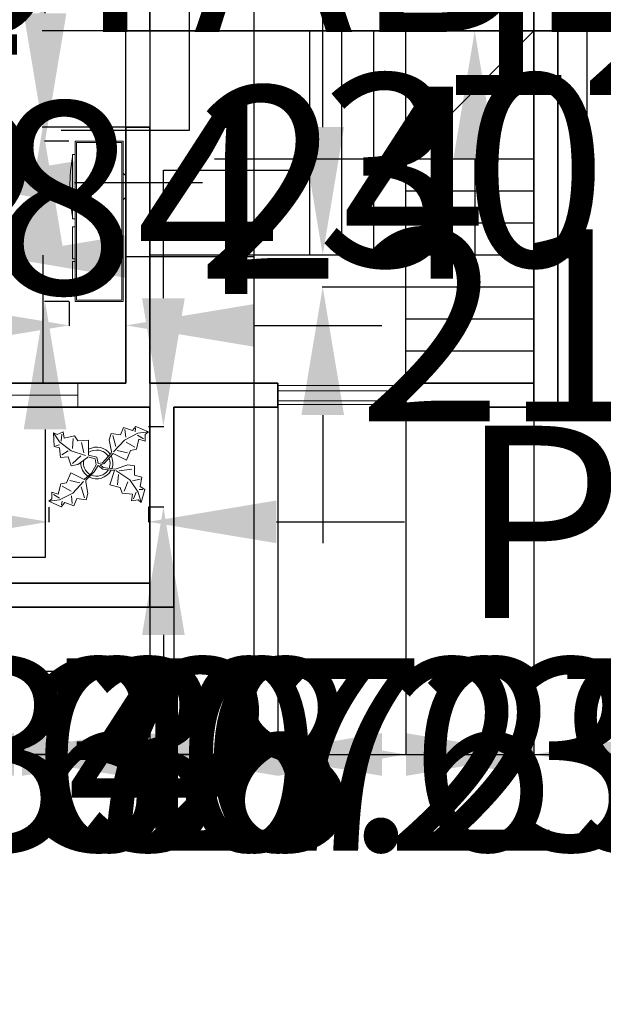
# Model space of a CAD drawing. Units: inches. Extents: x -307 to 2141, y -58 to 895.
# Tile 7 of 28: x 714 to 933, y -58 to 312. Entities that reach past the tile are written whole.
import ezdxf

# ---------------------------------------------------------------- set-up
doc = ezdxf.new("R2010")
doc.units = ezdxf.units.IN
doc.header["$MEASUREMENT"] = 0
for name, color, linetype, lineweight in [('A-ANNO-DIMS', 2, 'Continuous', 18), ('A-FLOR-STRS', 7, 'Continuous', 25), ('A-FURN', 8, 'Continuous', 18), ('A-GLAZ', 4, 'Continuous', 18), ('A-WALL', 7, 'Continuous', 35), ('L-PLNT', 94, 'Continuous', 13)]:
    doc.layers.add(name, color=color, linetype=linetype, lineweight=lineweight)
doc.styles.get("Standard").update_dxf_attribs({"font": 'arial.ttf'})
doc.dimstyles.get("Standard").update_dxf_attribs({"dimtxt": 72, "dimasz": 48, "dimexe": 0.18, "dimexo": 0.0625, "dimgap": 0.09, "dimtad": 0, "dimtih": 1, "dimtoh": 1, "dimdec": 0, "dimrnd": 48, "dimzin": 0, "dimdsep": 46, "dimlunit": 3, "dimtxsty": 'Standard', "dimcen": 0.09, "dimadec": 0, "dimazin": 0, "dimtfac": 1, "dimtdec": 0, "dimtofl": 0, "dimtmove": 0, "dimatfit": 3, "dimfxl": 1, "dimtolj": 1, "dimtzin": 0, "dimarcsym": 0})

# ---------------------------------------------------------------- blocks, each defined once
blk = doc.blocks.new('Entertainment Center')
for p, q in [((-4, 0), (-5, -1)), ((4, 0), (-4, 0)), ((5, -1), (4, 0)), ((-17, -19), (-17, -1)), ((-17, -1), (43, -1)), ((-16.5, -18.5), (-16.5, -1.5)), ((-16.5, -1.5), (42.5, -1.5)), ((42.5, -1.5), (42.5, -18.5)), ((43, -1), (43, -19)), ((43, -19), (-17, -19)), ((42.5, -18.5), (-16.5, -18.5)), ((-12, -20), (-12, -19)), ((12, -20), (-12, -20)), ((12, -19), (12, -20)), ((15, -20), (15, -19)), ((27, -20), (15, -20)), ((27, -19), (27, -20)), ((28, -20), (28, -19)), ((40, -20), (28, -20)), ((40, -19), (40, -20))]:
    blk.add_line(p, q)
blk.add_arc((0, 40), 61, 259.6111, 280.3889)
blk = doc.blocks.new('Plant - Rubber or Philodendron')
for p, q in [((-16.2005, 11.4774), (-13.9899, 8.1064)), ((-16.2005, 11.4774), (-14.8639, 10.7964)), ((-16.0159, 6.3329), (-16.2005, 11.4774)), ((-14.8639, 10.7964), (-12.6195, 11.8975)), ((-12.6195, 11.8975), (-12.1909, 9.4345)), ((4.6914, 8.8812), (5.3859, 11.2828)), ((5.3859, 11.2828), (8.8871, 10.7908)), ((8.8871, 10.7908), (9.9809, 13.4933)), ((9.9809, 13.4933), (13.3837, 12.301)), ((15.3859, 11.3055), (10.3916, 8.7942)), ((10.5828, 12.6946), (10.8893, 9.7953)), ((13.3837, 12.301), (14.68, 13.9039)), ((14.5816, 13.2037), (14.3848, 11.8033)), ((14.68, 13.9039), (19.3848, 11.8146)), ((19.3848, 11.8146), (15.3859, 11.3055)), ((19.3848, 11.8146), (18.1868, 10.9119)), ((-13.9899, 8.1064), (-9.5434, 4.7185)), ((-13.3174, 8.325), (-13.0735, 11.0065)), ((-12.1909, 9.4345), (-8.3829, 10.3)), ((-8.8369, 9.409), (-9.0894, 5.6095)), ((-8.3829, 10.3), (-7.0549, 8.501)), ((-7.0549, 8.501), (-3.0284, 8.6941)), ((-4.8529, 4.012), (-5.7184, 7.82)), ((-3.0284, 8.6941), (-3.0709, 3.1041)), ((4.6914, 8.8812), (5.5014, 4.4831)), ((5.9878, 10.4842), (7.1971, 6.3869)), ((10.3916, 8.7942), (6.2847, 4.4028)), ((14.2977, 6.1031), (10.9934, 7.9956)), ((15.7909, 9.1065), (14.8995, 5.3044)), ((15.2875, 10.6053), (17.5907, 9.2105)), ((18.1925, 8.4119), (15.7909, 9.1065)), ((18.1868, 10.9119), (18.1925, 8.4119)), ((-14.0069, 5.8704), (-16.0159, 6.3329)), ((-15.3434, 6.5514), (-13.9984, 6.9884)), ((-13.5868, 2.2894), (-14.0069, 5.8704)), ((-13.1329, 3.1804), (-10.6614, 4.727)), ((-9.5434, 4.7185), (-4.1917, 2.9888)), ((2.1141, 0.2298), (5.4346, 3.9146)), ((5.4346, 3.9146), (5.5014, 4.4831)), ((7.7005, 4.8881), (11.5025, 3.9967)), ((12.7005, 4.8994), (11.1089, 1.1958)), ((14.8995, 5.3044), (12.7005, 4.8994)), ((-10.6784, 2.491), (-13.5868, 2.2894)), ((-9.5858, -0.8715), (-10.6784, 2.491)), ((-9.1318, 0.0195), (-5.9793, 2.9025)), ((-7.1228, -0.443), (-3.5248, 2.2131)), ((-3.5248, 2.2131), (-3.3011, 2.4355)), ((-3.3011, 2.4355), (-0.5306, 1.7947)), ((-3.0709, 3.1041), (0.0797, 2.3163)), ((-0.5306, 1.7947), (-0.2255, -0.5527)), ((-0.5306, 1.7947), (-0.5306, 1.7947)), ((0.0797, 2.3163), (0.4866, -0.031)), ((0.4866, -0.031), (2.1141, 0.2298)), ((6.1032, 3.6844), (2.8262, -0.031)), ((11.1089, 1.1958), (6.1032, 3.6844)), ((-11.3237, -7.2629), (-9.7321, -3.5593)), ((-9.7321, -3.5593), (-4.7264, -6.0479)), ((-7.1228, -0.443), (-9.5858, -0.8715)), ((-2.019, -3.6148), (-4.7264, -6.0479)), ((-4.0579, -6.2781), (-0.9375, -3.1608)), ((-2.019, -3.6148), (-0.2255, -0.5527)), ((-0.9375, -3.1608), (0.5883, -0.8135)), ((0.5883, -0.8135), (2.2447, -2.0916)), ((2.8262, -0.031), (1.3003, -0.5527)), ((1.3003, -0.5527), (2.4193, -1.4655)), ((2.2447, -2.0916), (6.7108, -2.6626)), ((2.4193, -1.4655), (6.895, -2.1175)), ((4.943, -7.9659), (6.7108, -2.6626)), ((11.6605, -0.5413), (6.895, -2.1175)), ((12.3677, -6.1981), (7.219, -2.6772)), ((8.3544, -2.7453), (13.1973, -2.1704)), ((11.6605, -0.5413), (14.1354, -0.8948)), ((14.1354, -0.8948), (14.1354, -4.4304)), ((-13.5228, -7.6679), (-11.3237, -7.2629)), ((-6.3237, -7.2516), (-10.1257, -6.3602)), ((-9.0148, -11.1577), (-4.9047, -6.8122)), ((-4.1246, -6.8466), (-4.0579, -6.2781)), ((-3.3146, -11.2447), (-4.1246, -6.8466)), ((8.125, -4.0768), (7.7715, -7.9659)), ((10.2463, -10.4408), (11.6605, -6.9053)), ((15.5496, -10.7943), (12.3677, -6.1981)), ((16.2567, -5.8446), (13.4283, -6.5517)), ((14.1354, -4.4304), (16.9638, -5.1375)), ((16.9638, -5.1375), (16.2567, -8.673)), ((-16.8157, -10.7754), (-14.4141, -11.4699)), ((-16.8101, -13.2754), (-16.8157, -10.7754)), ((-14.4141, -11.4699), (-13.5228, -7.6679)), ((-12.921, -8.4665), (-9.6166, -10.359)), ((-4.611, -12.8477), (-5.8203, -8.7504)), ((8.8321, -9.0266), (4.943, -7.9659)), ((9.5392, -11.1479), (8.8321, -9.0266)), ((14.8425, -10.7943), (13.7819, -13.2692)), ((16.6103, -14.6834), (15.5496, -10.7943)), ((17.3174, -9.7337), (15.9032, -9.7337)), ((16.2567, -8.673), (18.0245, -9.7337)), ((18.0245, -9.7337), (16.6103, -14.6834)), ((-18.008, -14.1781), (-16.8101, -13.2754)), ((-18.008, -14.1781), (-14.0091, -13.669)), ((-13.3032, -16.2674), (-18.008, -14.1781)), ((-13.9107, -12.9688), (-16.2139, -11.574)), ((-14.0091, -13.669), (-9.0148, -11.1577)), ((-12.0069, -14.6645), (-13.3032, -16.2674)), ((-13.2048, -15.5672), (-13.008, -14.1668)), ((-8.6042, -15.8568), (-12.0069, -14.6645)), ((-9.206, -15.0581), (-9.5126, -12.1588)), ((-7.5103, -13.1543), (-8.6042, -15.8568)), ((-4.0092, -13.6463), (-7.5103, -13.1543)), ((-3.3146, -11.2447), (-4.0092, -13.6463)), ((13.4283, -11.5015), (9.5392, -11.1479)), ((13.0748, -13.9763), (13.4283, -11.5015)), ((15.5496, -13.6228), (13.0748, -13.9763)), ((16.6103, -14.6834), (15.5496, -13.6228))]:
    blk.add_line(p, q)
for centre, radius, start, end in [((0, 0), 6.1275, 34.37569, 120.1028), ((-0.0601, -0.2075), 5.2461, 33.82192, 124.9414), ((0.0308, 0.1664), 6, 178.6147, 235.1169), ((0.0308, 0.1664), 5, 168.1647, 238.6725), ((-0.2664, 0.1682), 5.2775, 338.4094, 20.03007), ((-0.098, 0.1364), 6.1288, 341.2017, 26.09184), ((-0.0234, 0.3825), 6.1492, 242.5812, 331.2714), ((-0.1102, 0.4886), 5.2883, 247.3711, 327.472)]:
    blk.add_arc(centre, radius, start, end)
blk = doc.blocks.new('WIN-36IN-PAIR')
for p, q in [((72.02, 9), (72.02, 0)), ((0, 4.5), (36, 4.5)), ((36.02, 4.5), (72.02, 4.5))]:
    blk.add_line(p, q)
for points in [[(36, 0), (0, 0), (0, 9), (36, 9)], [(36.02, 9), (72.02, 9)], [(72.02, 0), (36.02, 0)]]:
    blk.add_lwpolyline(points)
blk = doc.blocks.new('*D28')
at = {"layer": 'A-ANNO-DIMS', "color": 0, "lineweight": -2, "transparency": 16777216}
for p, q in [((795.36, 433.55), (777.92, 433.55)), ((778.1, 385.55), (778.1, 366.07)), ((795.36, 318.07), (777.92, 318.07)), ((778.1, 318.07), (778.1, 270.07)), ((778.1, 270.07), (730.1, 270.07))]:
    blk.add_line(p, q, dxfattribs=at)
at = {"layer": 'A-ANNO-DIMS', "color": 0, "transparency": 16777216}
for points in [[(770.1, 385.55), (786.1, 385.55), (778.1, 433.55)], [(770.1, 366.07), (786.1, 366.07), (778.1, 318.07)]]:
    blk.add_solid(points, dxfattribs=at)
at = {"layer": 'Defpoints', "color": 0, "transparency": 16777216}
for p in [(795.42, 433.55), (778.1, 318.07), (795.42, 318.07)]:
    blk.add_point(p, dxfattribs=at)
at = {"layer": 'A-ANNO-DIMS', "color": 0, "transparency": 16777216, "insert": (534.42, 270.07), "char_height": 72, "attachment_point": 5}
blk.add_mtext('\\A1;BED 115', dxfattribs=at)
blk = doc.blocks.new('*D34')
at = {"layer": 'A-ANNO-DIMS', "color": 0, "lineweight": -2, "transparency": 16777216}
for p, q in [((927.14, 490.97), (927.14, 538.97)), ((927.14, 538.97), (975.14, 538.97)), ((916.4, 442.97), (927.32, 442.97)), ((916.4, 370.95), (927.32, 370.95)), ((927.14, 322.95), (927.14, 274.95))]:
    blk.add_line(p, q, dxfattribs=at)
at = {"layer": 'A-ANNO-DIMS', "color": 0, "transparency": 16777216}
for points in [[(919.14, 490.97), (935.14, 490.97), (927.14, 442.97)], [(919.14, 322.95), (935.14, 322.95), (927.14, 370.95)]]:
    blk.add_solid(points, dxfattribs=at)
at = {"layer": 'Defpoints', "color": 0, "transparency": 16777216}
for p in [(916.34, 442.97), (927.14, 442.97), (916.34, 370.95)]:
    blk.add_point(p, dxfattribs=at)
at = {"layer": 'A-ANNO-DIMS', "color": 0, "transparency": 16777216, "insert": (1584.53, 538.97), "char_height": 72, "attachment_point": 5}
blk.add_mtext('\\A1;PAIRED WINDOW 72 TYP.', dxfattribs=at)
blk = doc.blocks.new('*D36')
at = {"layer": 'A-ANNO-DIMS', "color": 0, "lineweight": -2, "transparency": 16777216}
for p, q in [((871.71, 562.4), (871.76, 610.4)), ((876.55, 514.4), (871.47, 514.4)), ((876.51, 481.35), (871.44, 481.36)), ((871.56, 433.36), (871.51, 385.36)), ((871.51, 385.36), (823.51, 385.36))]:
    blk.add_line(p, q, dxfattribs=at)
at = {"layer": 'A-ANNO-DIMS', "color": 0, "transparency": 16777216}
for points in [[(863.71, 562.41), (879.71, 562.4), (871.65, 514.4)], [(863.56, 433.37), (879.56, 433.35), (871.62, 481.36)]]:
    blk.add_solid(points, dxfattribs=at)
at = {"layer": 'Defpoints', "color": 0, "transparency": 16777216}
for p in [(876.61, 514.4), (871.62, 481.36), (876.57, 481.35)]:
    blk.add_point(p, dxfattribs=at)
at = {"layer": 'A-ANNO-DIMS', "color": 0, "transparency": 16777216, "insert": (548.95, 385.36), "char_height": 72, "attachment_point": 5}
blk.add_mtext('\\A1;WC 33 TYP.', dxfattribs=at)
blk = doc.blocks.new('*D38')
at = {"layer": 'A-ANNO-DIMS', "color": 0, "lineweight": -2, "transparency": 16777216}
for p, q in [((598.5, 222.79), (550.5, 222.79)), ((646.5, 213.85), (646.5, 222.97)), ((706.5, 213.85), (706.5, 222.97)), ((754.5, 222.79), (802.5, 222.79))]:
    blk.add_line(p, q, dxfattribs=at)
at = {"layer": 'A-ANNO-DIMS', "color": 0, "transparency": 16777216}
for points in [[(598.5, 230.79), (598.5, 214.79), (646.5, 222.79)], [(754.5, 230.79), (754.5, 214.79), (706.5, 222.79)]]:
    blk.add_solid(points, dxfattribs=at)
at = {"layer": 'Defpoints', "color": 0, "transparency": 16777216}
for p in [(646.5, 222.79), (646.5, 213.79), (706.5, 213.79)]:
    blk.add_point(p, dxfattribs=at)
at = {"layer": 'A-ANNO-DIMS', "color": 0, "transparency": 16777216, "insert": (97.26, 222.79), "char_height": 72, "attachment_point": 5}
blk.add_mtext('\\A1;LOVESEAT 60 TYP.', dxfattribs=at)
blk = doc.blocks.new('*D40')
at = {"layer": 'A-ANNO-DIMS', "color": 0, "lineweight": -2, "transparency": 16777216}
for p, q in [((725.38, 128.89), (725.38, 123.17)), ((762.77, 128.89), (762.77, 123.17)), ((677.38, 123.35), (629.38, 123.35)), ((810.77, 123.35), (858.77, 123.35))]:
    blk.add_line(p, q, dxfattribs=at)
at = {"layer": 'A-ANNO-DIMS', "color": 0, "transparency": 16777216}
for points in [[(677.38, 131.35), (677.38, 115.35), (725.38, 123.35)], [(810.77, 131.35), (810.77, 115.35), (762.77, 123.35)]]:
    blk.add_solid(points, dxfattribs=at)
at = {"layer": 'Defpoints', "color": 0, "transparency": 16777216}
for p in [(725.38, 128.96), (762.77, 128.96), (762.77, 123.35)]:
    blk.add_point(p, dxfattribs=at)
at = {"layer": 'A-ANNO-DIMS', "color": 0, "transparency": 16777216, "insert": (1208.37, 123.35), "char_height": 72, "attachment_point": 5}
blk.add_mtext('\\A1;PLANT 37 TYP.', dxfattribs=at)
blk = doc.blocks.new('*D41')
at = {"layer": 'A-ANNO-DIMS', "color": 0, "lineweight": -2, "transparency": 16777216}
for p, q in [((768.38, 207.13), (768.38, 255.13)), ((768.38, 255.13), (816.38, 255.13)), ((762.83, 159.13), (768.56, 159.13)), ((762.83, 128.96), (768.56, 128.96)), ((768.38, 80.96), (768.38, 32.96))]:
    blk.add_line(p, q, dxfattribs=at)
at = {"layer": 'A-ANNO-DIMS', "color": 0, "transparency": 16777216}
for points in [[(760.38, 207.13), (776.38, 207.13), (768.38, 159.13)], [(760.38, 80.96), (776.38, 80.96), (768.38, 128.96)]]:
    blk.add_solid(points, dxfattribs=at)
at = {"layer": 'Defpoints', "color": 0, "transparency": 16777216}
for p in [(762.77, 159.13), (768.38, 159.13), (762.77, 128.96)]:
    blk.add_point(p, dxfattribs=at)
at = {"layer": 'A-ANNO-DIMS', "color": 0, "transparency": 16777216, "insert": (991.68, 255.13), "char_height": 72, "attachment_point": 5}
blk.add_mtext('\\A1;30 TYP.', dxfattribs=at)
blk = doc.blocks.new('*D48')
at = {"layer": 'A-ANNO-DIMS', "color": 0, "lineweight": -2, "transparency": 16777216}
for p, q in [((724, 313.98), (724, 361.98)), ((732.94, 265.98), (723.82, 265.98)), ((732.94, 205.98), (723.82, 205.98)), ((724, 157.98), (724, 109.98)), ((724, 109.98), (676, 109.98))]:
    blk.add_line(p, q, dxfattribs=at)
at = {"layer": 'A-ANNO-DIMS', "color": 0, "transparency": 16777216}
for points in [[(716, 313.98), (732, 313.98), (724, 265.98)], [(716, 157.98), (732, 157.98), (724, 205.98)]]:
    blk.add_solid(points, dxfattribs=at)
at = {"layer": 'Defpoints', "color": 0, "transparency": 16777216}
for p in [(733, 265.98), (724, 205.98), (733, 205.98)]:
    blk.add_point(p, dxfattribs=at)
at = {"layer": 'A-ANNO-DIMS', "color": 0, "transparency": 16777216, "insert": (321.56, 109.98), "char_height": 72, "attachment_point": 5}
blk.add_mtext('\\A1;MEDIA UNIT 60', dxfattribs=at)
blk = doc.blocks.new('*D49')
at = {"layer": 'A-ANNO-DIMS', "color": 0, "lineweight": -2, "transparency": 16777216}
for p, q in [((733, 205.92), (733, 196.8)), ((754.34, 205.92), (754.34, 196.8)), ((685, 196.98), (637, 196.98)), ((802.34, 196.98), (850.34, 196.98))]:
    blk.add_line(p, q, dxfattribs=at)
at = {"layer": 'A-ANNO-DIMS', "color": 0, "transparency": 16777216}
for points in [[(685, 204.98), (685, 188.98), (733, 196.98)], [(802.34, 204.98), (802.34, 188.98), (754.34, 196.98)]]:
    blk.add_solid(points, dxfattribs=at)
at = {"layer": 'Defpoints', "color": 0, "transparency": 16777216}
for p in [(733, 205.98), (754.34, 205.98), (754.34, 196.98)]:
    blk.add_point(p, dxfattribs=at)
at = {"layer": 'A-ANNO-DIMS', "color": 0, "transparency": 16777216, "insert": (895.66, 196.98), "char_height": 72, "attachment_point": 5}
blk.add_mtext('\\A1;21', dxfattribs=at)
blk = doc.blocks.new('*D52')
at = {"layer": 'A-ANNO-DIMS', "color": 0, "lineweight": -2, "transparency": 16777216}
for p, q in [((660.21, 554.25), (660.21, 602.25)), ((673.8, 506.25), (660.03, 506.25)), ((673.8, 415.25), (660.03, 415.25)), ((660.21, 367.25), (660.21, 319.25))]:
    blk.add_line(p, q, dxfattribs=at)
at = {"layer": 'A-ANNO-DIMS', "color": 0, "transparency": 16777216}
for points in [[(652.21, 554.25), (668.21, 554.25), (660.21, 506.25)], [(652.21, 367.25), (668.21, 367.25), (660.21, 415.25)]]:
    blk.add_solid(points, dxfattribs=at)
at = {"layer": 'Defpoints', "color": 0, "transparency": 16777216}
for p in [(673.86, 506.25), (660.21, 415.25), (673.86, 415.25)]:
    blk.add_point(p, dxfattribs=at)
at = {"layer": 'A-ANNO-DIMS', "color": 0, "transparency": 16777216, "insert": (660.21, 460.75), "char_height": 72, "attachment_point": 5}
blk.add_mtext('\\A1;DINING SET 91', dxfattribs=at)
blk = doc.blocks.new('*D54')
at = {"layer": 'A-ANNO-DIMS', "color": 0, "lineweight": -2, "transparency": 16777216}
for p, q in [((605.34, 412.35), (605.34, 460.35)), ((605.34, 460.35), (653.34, 460.35)), ((596.4, 364.35), (605.52, 364.35)), ((596.4, 304.35), (605.52, 304.35)), ((605.34, 256.35), (605.34, 208.35))]:
    blk.add_line(p, q, dxfattribs=at)
at = {"layer": 'A-ANNO-DIMS', "color": 0, "transparency": 16777216}
for points in [[(597.34, 412.35), (613.34, 412.35), (605.34, 364.35)], [(597.34, 256.35), (613.34, 256.35), (605.34, 304.35)]]:
    blk.add_solid(points, dxfattribs=at)
at = {"layer": 'Defpoints', "color": 0, "transparency": 16777216}
for p in [(596.34, 364.35), (605.34, 364.35), (596.34, 304.35)]:
    blk.add_point(p, dxfattribs=at)
at = {"layer": 'A-ANNO-DIMS', "color": 0, "transparency": 16777216, "insert": (854, 460.35), "char_height": 72, "attachment_point": 5}
blk.add_mtext('\\A1;DESK 60', dxfattribs=at)
blk = doc.blocks.new('*D58')
at = {"layer": 'A-ANNO-DIMS', "color": 0, "lineweight": -2, "transparency": 16777216}
for p, q in [((624.38, 334.8), (624.38, 382.8)), ((611.84, 286.8), (624.56, 286.8)), ((611.84, 202.8), (624.56, 202.8)), ((624.38, 154.8), (624.38, 106.8))]:
    blk.add_line(p, q, dxfattribs=at)
at = {"layer": 'A-ANNO-DIMS', "color": 0, "transparency": 16777216}
for points in [[(616.38, 334.8), (632.38, 334.8), (624.38, 286.8)], [(616.38, 154.8), (632.38, 154.8), (624.38, 202.8)]]:
    blk.add_solid(points, dxfattribs=at)
at = {"layer": 'Defpoints', "color": 0, "transparency": 16777216}
for p in [(611.78, 286.8), (624.38, 286.8), (611.78, 202.8)]:
    blk.add_point(p, dxfattribs=at)
at = {"layer": 'A-ANNO-DIMS', "color": 0, "transparency": 16777216, "insert": (624.38, 244.8), "char_height": 72, "attachment_point": 5}
blk.add_mtext('\\A1;SOFA 84', dxfattribs=at)
blk = doc.blocks.new('*D60')
at = {"layer": 'A-ANNO-DIMS', "color": 0, "lineweight": -2, "transparency": 16777216}
for p, q in [((659.86, 294.95), (659.86, 342.95)), ((659.86, 342.95), (707.86, 342.95)), ((663.34, 246.95), (659.68, 246.95)), ((663.34, 223.32), (659.68, 223.32)), ((659.86, 175.32), (659.86, 127.32))]:
    blk.add_line(p, q, dxfattribs=at)
at = {"layer": 'A-ANNO-DIMS', "color": 0, "transparency": 16777216}
for points in [[(651.86, 294.95), (667.86, 294.95), (659.86, 246.95)], [(651.86, 175.32), (667.86, 175.32), (659.86, 223.32)]]:
    blk.add_solid(points, dxfattribs=at)
at = {"layer": 'Defpoints', "color": 0, "transparency": 16777216}
for p in [(659.86, 246.95), (663.4, 246.95), (663.4, 223.32)]:
    blk.add_point(p, dxfattribs=at)
at = {"layer": 'A-ANNO-DIMS', "color": 0, "transparency": 16777216, "insert": (933.57, 342.95), "char_height": 72, "attachment_point": 5}
blk.add_mtext('\\A1;TABLE 24', dxfattribs=at)
blk = doc.blocks.new('*D61')
at = {"layer": 'A-ANNO-DIMS', "color": 0, "lineweight": -2, "transparency": 16777216}
for p, q in [((615.4, 250.49), (567.4, 250.49)), ((663.4, 247.01), (663.4, 250.67)), ((687.03, 247.01), (687.03, 250.67)), ((735.03, 250.49), (783.03, 250.49))]:
    blk.add_line(p, q, dxfattribs=at)
at = {"layer": 'A-ANNO-DIMS', "color": 0, "transparency": 16777216}
for points in [[(615.4, 258.49), (615.4, 242.49), (663.4, 250.49)], [(735.03, 258.49), (735.03, 242.49), (687.03, 250.49)]]:
    blk.add_solid(points, dxfattribs=at)
at = {"layer": 'Defpoints', "color": 0, "transparency": 16777216}
for p in [(687.03, 250.49), (663.4, 246.95), (687.03, 246.95)]:
    blk.add_point(p, dxfattribs=at)
at = {"layer": 'A-ANNO-DIMS', "color": 0, "transparency": 16777216, "insert": (835.16, 250.49), "char_height": 72, "attachment_point": 5}
blk.add_mtext('\\A1;24', dxfattribs=at)
blk = doc.blocks.new('*D63')
at = {"layer": 'A-ANNO-DIMS', "color": 0, "lineweight": -2, "transparency": 16777216}
for p, q in [((916.4, 691.34), (947.72, 691.34)), ((947.54, 643.34), (947.54, 416.19)), ((947.54, 115.34), (947.54, 342.49)), ((704.68, 67.34), (947.72, 67.34))]:
    blk.add_line(p, q, dxfattribs=at)
at = {"layer": 'A-ANNO-DIMS', "color": 0, "transparency": 16777216}
for points in [[(939.54, 643.34), (955.54, 643.34), (947.54, 691.34)], [(939.54, 115.34), (955.54, 115.34), (947.54, 67.34)]]:
    blk.add_solid(points, dxfattribs=at)
at = {"layer": 'Defpoints', "color": 0, "transparency": 16777216}
for p in [(916.34, 691.34), (704.62, 67.34), (947.54, 67.34)]:
    blk.add_point(p, dxfattribs=at)
at = {"layer": 'A-ANNO-DIMS', "color": 0, "transparency": 16777216, "insert": (947.54, 379.34), "char_height": 72, "attachment_point": 5}
blk.add_mtext('\\A1;624', dxfattribs=at)
blk = doc.blocks.new('*D72')
at = {"layer": 'A-ANNO-DIMS', "color": 0, "lineweight": -2, "transparency": 16777216}
for p, q in [((556.34, 91.28), (556.34, 35.96)), ((632.62, 91.28), (632.62, 35.96)), ((508.34, 36.14), (460.34, 36.14)), ((680.62, 36.14), (728.62, 36.14))]:
    blk.add_line(p, q, dxfattribs=at)
at = {"layer": 'A-ANNO-DIMS', "color": 0, "transparency": 16777216}
for points in [[(508.34, 44.14), (508.34, 28.14), (556.34, 36.14)], [(680.62, 44.14), (680.62, 28.14), (632.62, 36.14)]]:
    blk.add_solid(points, dxfattribs=at)
at = {"layer": 'Defpoints', "color": 0, "transparency": 16777216}
for p in [(556.34, 91.34), (632.62, 91.34), (632.62, 36.14)]:
    blk.add_point(p, dxfattribs=at)
at = {"layer": 'A-ANNO-DIMS', "color": 0, "transparency": 16777216, "insert": (849.97, 36.14), "char_height": 72, "attachment_point": 5}
blk.add_mtext('\\A1;76.29', dxfattribs=at)
blk = doc.blocks.new('*D73')
at = {"layer": 'A-ANNO-DIMS', "color": 0, "lineweight": -2, "transparency": 16777216}
for p, q in [((632.62, 91.28), (632.62, 35.96)), ((704.62, 91.28), (704.62, 35.96)), ((584.62, 36.14), (536.62, 36.14)), ((752.62, 36.14), (800.62, 36.14))]:
    blk.add_line(p, q, dxfattribs=at)
at = {"layer": 'A-ANNO-DIMS', "color": 0, "transparency": 16777216}
for points in [[(584.62, 44.14), (584.62, 28.14), (632.62, 36.14)], [(752.62, 44.14), (752.62, 28.14), (704.62, 36.14)]]:
    blk.add_solid(points, dxfattribs=at)
at = {"layer": 'Defpoints', "color": 0, "transparency": 16777216}
for p in [(632.62, 91.34), (704.62, 91.34), (704.62, 36.14)]:
    blk.add_point(p, dxfattribs=at)
at = {"layer": 'A-ANNO-DIMS', "color": 0, "transparency": 16777216, "insert": (851.62, 36.14), "char_height": 72, "attachment_point": 5}
blk.add_mtext('\\A1;72', dxfattribs=at)
blk = doc.blocks.new('*D74')
at = {"layer": 'A-ANNO-DIMS', "color": 0, "lineweight": -2, "transparency": 16777216}
for p, q in [((704.62, 91.28), (704.62, 35.96)), ((772.34, 91.28), (772.34, 35.96)), ((656.62, 36.14), (608.62, 36.14)), ((820.34, 36.14), (868.34, 36.14))]:
    blk.add_line(p, q, dxfattribs=at)
at = {"layer": 'A-ANNO-DIMS', "color": 0, "transparency": 16777216}
for points in [[(656.62, 44.14), (656.62, 28.14), (704.62, 36.14)], [(820.34, 44.14), (820.34, 28.14), (772.34, 36.14)]]:
    blk.add_solid(points, dxfattribs=at)
at = {"layer": 'Defpoints', "color": 0, "transparency": 16777216}
for p in [(704.62, 91.34), (772.34, 91.34), (772.34, 36.14)]:
    blk.add_point(p, dxfattribs=at)
at = {"layer": 'A-ANNO-DIMS', "color": 0, "transparency": 16777216, "insert": (983.15, 36.14), "char_height": 72, "attachment_point": 5}
blk.add_mtext('\\A1;67.71', dxfattribs=at)
blk = doc.blocks.new('*D84')
at = {"layer": 'A-ANNO-DIMS', "color": 0, "lineweight": -2, "transparency": 16777216}
for p, q in [((763.34, 472.28), (763.34, 35.96)), ((907.34, 472.28), (907.34, 35.96)), ((811.34, 36.14), (859.34, 36.14)), ((907.34, 36.14), (955.34, 36.14))]:
    blk.add_line(p, q, dxfattribs=at)
at = {"layer": 'A-ANNO-DIMS', "color": 0, "transparency": 16777216}
for points in [[(811.34, 44.14), (811.34, 28.14), (763.34, 36.14)], [(859.34, 44.14), (859.34, 28.14), (907.34, 36.14)]]:
    blk.add_solid(points, dxfattribs=at)
at = {"layer": 'Defpoints', "color": 0, "transparency": 16777216}
for p in [(763.34, 472.34), (907.34, 472.34), (907.34, 36.14)]:
    blk.add_point(p, dxfattribs=at)
at = {"layer": 'A-ANNO-DIMS', "color": 0, "transparency": 16777216, "insert": (1031.43, 36.14), "char_height": 72, "attachment_point": 5}
blk.add_mtext('\\A1;144', dxfattribs=at)
blk = doc.blocks.new('*D86')
at = {"layer": 'A-ANNO-DIMS', "color": 0, "lineweight": -2, "transparency": 16777216}
for p, q in [((565.34, 304.28), (565.34, 35.96)), ((625.34, 304.28), (625.34, 35.96)), ((517.34, 36.14), (469.34, 36.14)), ((673.34, 36.14), (721.34, 36.14))]:
    blk.add_line(p, q, dxfattribs=at)
at = {"layer": 'A-ANNO-DIMS', "color": 0, "transparency": 16777216}
for points in [[(517.34, 44.14), (517.34, 28.14), (565.34, 36.14)], [(673.34, 44.14), (673.34, 28.14), (625.34, 36.14)]]:
    blk.add_solid(points, dxfattribs=at)
at = {"layer": 'Defpoints', "color": 0, "transparency": 16777216}
for p in [(565.34, 304.34), (625.34, 304.34), (625.34, 36.14)]:
    blk.add_point(p, dxfattribs=at)
at = {"layer": 'A-ANNO-DIMS', "color": 0, "transparency": 16777216, "insert": (773.07, 36.14), "char_height": 72, "attachment_point": 5}
blk.add_mtext('\\A1;60', dxfattribs=at)
blk = doc.blocks.new('*D88')
at = {"layer": 'A-ANNO-DIMS', "color": 0, "lineweight": -2, "transparency": 16777216}
for p, q in [((517.33584, 722.544828), (469.33584, 722.544828)), ((565.33584, 295.403328), (565.33584, 722.724828)), ((754.33584, 271.403328), (754.33584, 722.724828)), ((802.33584, 722.544828), (850.33584, 722.544828))]:
    blk.add_line(p, q, dxfattribs=at)
at = {"layer": 'A-ANNO-DIMS', "color": 0, "transparency": 16777216}
for points in [[(517.33584, 730.544828), (517.33584, 714.544828), (565.33584, 722.544828)], [(802.33584, 730.544828), (802.33584, 714.544828), (754.33584, 722.544828)]]:
    blk.add_solid(points, dxfattribs=at)
at = {"layer": 'Defpoints', "color": 0, "transparency": 16777216}
for p in [(754.33584, 722.544828), (565.33584, 295.340828), (754.33584, 271.340828)]:
    blk.add_point(p, dxfattribs=at)
at = {"layer": 'A-ANNO-DIMS', "color": 0, "transparency": 16777216, "insert": (659.83584, 722.544828), "char_height": 72, "attachment_point": 5}
blk.add_mtext('\\A1;189', dxfattribs=at)
blk = doc.blocks.new('*D89')
at = {"layer": 'A-ANNO-DIMS', "color": 0, "lineweight": -2, "transparency": 16777216}
for p, q in [((525.13, 295.34), (525.13, 343.34)), ((525.13, 343.34), (573.13, 343.34)), ((565.27, 295.34), (524.95, 295.34)), ((525.13, 223.34), (525.13, 247.34)), ((556.27, 175.34), (524.95, 175.34))]:
    blk.add_line(p, q, dxfattribs=at)
at = {"layer": 'A-ANNO-DIMS', "color": 0, "transparency": 16777216}
for points in [[(517.13, 247.34), (533.13, 247.34), (525.13, 295.34)], [(517.13, 223.34), (533.13, 223.34), (525.13, 175.34)]]:
    blk.add_solid(points, dxfattribs=at)
at = {"layer": 'Defpoints', "color": 0, "transparency": 16777216}
for p in [(525.13, 295.34), (565.34, 295.34), (556.34, 175.34)]:
    blk.add_point(p, dxfattribs=at)
at = {"layer": 'A-ANNO-DIMS', "color": 0, "transparency": 16777216, "insert": (649.25, 343.34), "char_height": 72, "attachment_point": 5}
blk.add_mtext('\\A1;120', dxfattribs=at)
blk = doc.blocks.new('*D90')
at = {"layer": 'A-ANNO-DIMS', "color": 0, "lineweight": -2, "transparency": 16777216}
for p, q in [((556.34, 166.28), (556.34, 35.96)), ((589.34, 166.28), (589.34, 35.96)), ((508.34, 36.14), (460.34, 36.14)), ((637.34, 36.14), (685.34, 36.14))]:
    blk.add_line(p, q, dxfattribs=at)
at = {"layer": 'A-ANNO-DIMS', "color": 0, "transparency": 16777216}
for points in [[(508.34, 44.14), (508.34, 28.14), (556.34, 36.14)], [(637.34, 44.14), (637.34, 28.14), (589.34, 36.14)]]:
    blk.add_solid(points, dxfattribs=at)
at = {"layer": 'Defpoints', "color": 0, "transparency": 16777216}
for p in [(556.34, 166.34), (589.34, 166.34), (589.34, 36.14)]:
    blk.add_point(p, dxfattribs=at)
at = {"layer": 'A-ANNO-DIMS', "color": 0, "transparency": 16777216, "insert": (736.97, 36.14), "char_height": 72, "attachment_point": 5}
blk.add_mtext('\\A1;33', dxfattribs=at)
blk = doc.blocks.new('*D91')
at = {"layer": 'A-ANNO-DIMS', "color": 0, "lineweight": -2, "transparency": 16777216}
for p, q in [((589.34, 166.28), (589.34, 35.96)), ((637.34, 166.28), (637.34, 35.96)), ((541.34, 36.14), (493.34, 36.14)), ((685.34, 36.14), (733.34, 36.14))]:
    blk.add_line(p, q, dxfattribs=at)
at = {"layer": 'A-ANNO-DIMS', "color": 0, "transparency": 16777216}
for points in [[(541.34, 44.14), (541.34, 28.14), (589.34, 36.14)], [(685.34, 44.14), (685.34, 28.14), (637.34, 36.14)]]:
    blk.add_solid(points, dxfattribs=at)
at = {"layer": 'Defpoints', "color": 0, "transparency": 16777216}
for p in [(589.34, 166.34), (637.34, 166.34), (637.34, 36.14)]:
    blk.add_point(p, dxfattribs=at)
at = {"layer": 'A-ANNO-DIMS', "color": 0, "transparency": 16777216, "insert": (786.52, 36.14), "char_height": 72, "attachment_point": 5}
blk.add_mtext('\\A1;48', dxfattribs=at)
blk = doc.blocks.new('*D92')
at = {"layer": 'A-ANNO-DIMS', "color": 0, "lineweight": -2, "transparency": 16777216}
for p, q in [((637.34, 166.28), (637.34, 35.96)), ((664.34, 166.28), (664.34, 35.96)), ((589.34, 36.14), (541.34, 36.14)), ((712.34, 36.14), (760.34, 36.14))]:
    blk.add_line(p, q, dxfattribs=at)
at = {"layer": 'A-ANNO-DIMS', "color": 0, "transparency": 16777216}
for points in [[(589.34, 44.14), (589.34, 28.14), (637.34, 36.14)], [(712.34, 44.14), (712.34, 28.14), (664.34, 36.14)]]:
    blk.add_solid(points, dxfattribs=at)
at = {"layer": 'Defpoints', "color": 0, "transparency": 16777216}
for p in [(637.34, 166.34), (664.34, 166.34), (664.34, 36.14)]:
    blk.add_point(p, dxfattribs=at)
at = {"layer": 'A-ANNO-DIMS', "color": 0, "transparency": 16777216, "insert": (812.61, 36.14), "char_height": 72, "attachment_point": 5}
blk.add_mtext('\\A1;27', dxfattribs=at)
blk = doc.blocks.new('*D93')
at = {"layer": 'A-ANNO-DIMS', "color": 0, "lineweight": -2, "transparency": 16777216}
for p, q in [((859.34, 175.28), (859.34, 35.96)), ((907.34, 175.28), (907.34, 35.96)), ((811.34, 36.14), (763.34, 36.14)), ((955.34, 36.14), (1003.34, 36.14))]:
    blk.add_line(p, q, dxfattribs=at)
at = {"layer": 'A-ANNO-DIMS', "color": 0, "transparency": 16777216}
for points in [[(811.34, 44.14), (811.34, 28.14), (859.34, 36.14)], [(955.34, 44.14), (955.34, 28.14), (907.34, 36.14)]]:
    blk.add_solid(points, dxfattribs=at)
at = {"layer": 'Defpoints', "color": 0, "transparency": 16777216}
for p in [(859.34, 175.34), (907.34, 175.34), (907.34, 36.14)]:
    blk.add_point(p, dxfattribs=at)
at = {"layer": 'A-ANNO-DIMS', "color": 0, "transparency": 16777216, "insert": (1056.52, 36.14), "char_height": 72, "attachment_point": 5}
blk.add_mtext('\\A1;48', dxfattribs=at)
blk = doc.blocks.new('*D99')
at = {"layer": 'A-ANNO-DIMS', "color": 0, "lineweight": -2, "transparency": 16777216}
for p, q in [((763.34, 481.28), (763.34, 35.96)), ((802.34, 481.28), (802.34, 35.96)), ((715.34, 36.14), (667.34, 36.14)), ((850.34, 36.14), (898.34, 36.14))]:
    blk.add_line(p, q, dxfattribs=at)
at = {"layer": 'A-ANNO-DIMS', "color": 0, "transparency": 16777216}
for points in [[(715.34, 44.14), (715.34, 28.14), (763.34, 36.14)], [(850.34, 44.14), (850.34, 28.14), (802.34, 36.14)]]:
    blk.add_solid(points, dxfattribs=at)
at = {"layer": 'Defpoints', "color": 0, "transparency": 16777216}
for p in [(763.34, 481.34), (802.34, 481.34), (802.34, 36.14)]:
    blk.add_point(p, dxfattribs=at)
at = {"layer": 'A-ANNO-DIMS', "color": 0, "transparency": 16777216, "insert": (950.04, 36.14), "char_height": 72, "attachment_point": 5}
blk.add_mtext('\\A1;39', dxfattribs=at)
blk = doc.blocks.new('*D100')
at = {"layer": 'A-ANNO-DIMS', "color": 0, "lineweight": -2, "transparency": 16777216}
for p, q in [((589.34, 409.28), (589.34, 35.96)), ((625.34, 409.28), (625.34, 35.96)), ((541.34, 36.14), (493.34, 36.14)), ((673.34, 36.14), (721.34, 36.14))]:
    blk.add_line(p, q, dxfattribs=at)
at = {"layer": 'A-ANNO-DIMS', "color": 0, "transparency": 16777216}
for points in [[(541.34, 44.14), (541.34, 28.14), (589.34, 36.14)], [(673.34, 44.14), (673.34, 28.14), (625.34, 36.14)]]:
    blk.add_solid(points, dxfattribs=at)
at = {"layer": 'Defpoints', "color": 0, "transparency": 16777216}
for p in [(589.34, 409.34), (625.34, 409.34), (625.34, 36.14)]:
    blk.add_point(p, dxfattribs=at)
at = {"layer": 'A-ANNO-DIMS', "color": 0, "transparency": 16777216, "insert": (772.95, 36.14), "char_height": 72, "attachment_point": 5}
blk.add_mtext('\\A1;36', dxfattribs=at)
blk = doc.blocks.new('*D104')
at = {"layer": 'A-ANNO-DIMS', "color": 0, "lineweight": -2, "transparency": 16777216}
for p, q in [((885.13, 418.95), (885.13, 466.95)), ((885.13, 466.95), (933.13, 466.95)), ((916.27, 370.95), (884.95, 370.95)), ((916.27, 307.34), (884.95, 307.34)), ((885.13, 259.34), (885.13, 211.34))]:
    blk.add_line(p, q, dxfattribs=at)
at = {"layer": 'A-ANNO-DIMS', "color": 0, "transparency": 16777216}
for points in [[(877.13, 418.95), (893.13, 418.95), (885.13, 370.95)], [(877.13, 259.34), (893.13, 259.34), (885.13, 307.34)]]:
    blk.add_solid(points, dxfattribs=at)
at = {"layer": 'Defpoints', "color": 0, "transparency": 16777216}
for p in [(885.13, 370.95), (916.34, 370.95), (916.34, 307.34)]:
    blk.add_point(p, dxfattribs=at)
at = {"layer": 'A-ANNO-DIMS', "color": 0, "transparency": 16777216, "insert": (1047.95, 466.95), "char_height": 72, "attachment_point": 5}
blk.add_mtext('\\A1;63.61', dxfattribs=at)
blk = doc.blocks.new('*D105')
at = {"layer": 'A-ANNO-DIMS', "color": 0, "lineweight": -2, "transparency": 16777216}
for p, q in [((828.13, 271.34), (828.13, 319.34)), ((828.13, 319.34), (876.13, 319.34)), ((859.27, 223.34), (827.95, 223.34)), ((859.27, 211.34), (827.95, 211.34)), ((828.13, 163.34), (828.13, 115.34))]:
    blk.add_line(p, q, dxfattribs=at)
at = {"layer": 'A-ANNO-DIMS', "color": 0, "transparency": 16777216}
for points in [[(820.13, 271.34), (836.13, 271.34), (828.13, 223.34)], [(820.13, 163.34), (836.13, 163.34), (828.13, 211.34)]]:
    blk.add_solid(points, dxfattribs=at)
at = {"layer": 'Defpoints', "color": 0, "transparency": 16777216}
for p in [(828.13, 223.34), (859.34, 223.34), (859.34, 211.34)]:
    blk.add_point(p, dxfattribs=at)
at = {"layer": 'A-ANNO-DIMS', "color": 0, "transparency": 16777216, "insert": (924.03, 319.34), "char_height": 72, "attachment_point": 5}
blk.add_mtext('\\A1;12', dxfattribs=at)
blk = doc.blocks.new('*D106')
at = {"layer": 'A-ANNO-DIMS', "color": 0, "lineweight": -2, "transparency": 16777216}
for p, q in [((811.34, 166.28), (811.34, 35.96)), ((859.34, 166.28), (859.34, 35.96)), ((763.34, 36.14), (715.34, 36.14)), ((907.34, 36.14), (955.34, 36.14))]:
    blk.add_line(p, q, dxfattribs=at)
at = {"layer": 'A-ANNO-DIMS', "color": 0, "transparency": 16777216}
for points in [[(763.34, 44.14), (763.34, 28.14), (811.34, 36.14)], [(907.34, 44.14), (907.34, 28.14), (859.34, 36.14)]]:
    blk.add_solid(points, dxfattribs=at)
at = {"layer": 'Defpoints', "color": 0, "transparency": 16777216}
for p in [(811.34, 166.34), (859.34, 166.34), (859.34, 36.14)]:
    blk.add_point(p, dxfattribs=at)
at = {"layer": 'A-ANNO-DIMS', "color": 0, "transparency": 16777216, "insert": (1008.52, 36.14), "char_height": 72, "attachment_point": 5}
blk.add_mtext('\\A1;48', dxfattribs=at)
blk = doc.blocks.new('*D109')
at = {"layer": 'A-ANNO-DIMS', "color": 0, "lineweight": -2, "transparency": 16777216}
for p, q in [((723.13, 355.34), (723.13, 403.34)), ((723.13, 403.34), (771.13, 403.34)), ((754.27, 307.34), (722.95, 307.34)), ((754.27, 271.34), (722.95, 271.34)), ((723.13, 223.34), (723.13, 175.34))]:
    blk.add_line(p, q, dxfattribs=at)
at = {"layer": 'A-ANNO-DIMS', "color": 0, "transparency": 16777216}
for points in [[(715.13, 355.34), (731.13, 355.34), (723.13, 307.34)], [(715.13, 223.34), (731.13, 223.34), (723.13, 271.34)]]:
    blk.add_solid(points, dxfattribs=at)
at = {"layer": 'Defpoints', "color": 0, "transparency": 16777216}
for p in [(723.13, 307.34), (754.34, 307.34), (754.34, 271.34)]:
    blk.add_point(p, dxfattribs=at)
at = {"layer": 'A-ANNO-DIMS', "color": 0, "transparency": 16777216, "insert": (822.74, 403.34), "char_height": 72, "attachment_point": 5}
blk.add_mtext('\\A1;36', dxfattribs=at)

msp = doc.modelspace()

# ---------------------------------------------------------------- linework, layer by layer
at = {"layer": 'A-FLOR-STRS'}
for p, q in [((847.3358, 307.3408), (787.4974, 307.3408)), ((823.3358, 223.3408), (823.3358, 307.3408)), ((835.3358, 223.3408), (835.3358, 307.3408)), ((907.3358, 307.3408), (847.3358, 307.3408)), ((847.3358, 223.3408), (847.3358, 307.3408)), ((859.3358, 166.3408), (859.3358, 307.3408)), ((907.3358, 307.3408), (859.3358, 259.3408)), ((907.3358, 307.3408), (907.3358, 166.3408)), ((907.3358, 166.3408), (907.3358, 307.3408)), ((859.3358, 259.3408), (787.4974, 259.3408)), ((907.3358, 259.3408), (859.3358, 259.3408)), ((907.3358, 247.3408), (859.3358, 247.3408)), ((907.3358, 235.3408), (859.3358, 235.3408)), ((859.3358, 223.3408), (763.3358, 223.3408)), ((907.3358, 223.3408), (859.3358, 223.3408)), ((907.3358, 211.3408), (859.3358, 211.3408)), ((907.3358, 199.3408), (859.3358, 199.3408)), ((907.3358, 187.3408), (859.3358, 187.3408)), ((907.3358, 175.3408), (859.3358, 175.3408)), ((907.3358, 175.3408), (859.3358, 175.3408))]:
    msp.add_line(p, q, dxfattribs=at)
at = {"layer": 'A-GLAZ'}
for p, q in [((859.3358, 174.3952), (811.3358, 174.3952)), ((859.3358, 172.4884), (811.3358, 172.4884)), ((859.3358, 168.6586), (811.3358, 168.6586)), ((859.3358, 167.2864), (811.3358, 167.2864))]:
    msp.add_line(p, q, dxfattribs=at)
at = {"layer": 'A-WALL'}
for p, q in [((916.3358, 166.3408), (916.3358, 691.3408)), ((907.3358, 166.3408), (907.3358, 682.3408)), ((754.3358, 307.3408), (754.3358, 481.3408)), ((754.3358, 307.3408), (754.3358, 481.3408)), ((763.3358, 307.3408), (763.3358, 481.3408)), ((763.3358, 307.3408), (763.3358, 481.3408)), ((916.3358, 307.3408), (754.3358, 307.3408)), ((763.3358, 271.3408), (754.3358, 271.3408)), ((754.3358, 175.3408), (754.3358, 271.3408)), ((763.3358, 175.3408), (763.3358, 271.3408)), ((754.3358, 175.3408), (637.3358, 175.3408)), ((811.3358, 175.3408), (763.3358, 175.3408)), ((811.3358, 166.3408), (811.3358, 175.3408)), ((907.3358, 175.3408), (859.3358, 175.3408)), ((763.3358, 166.3408), (637.3358, 166.3408)), ((763.3358, 166.3408), (763.3358, 100.3408)), ((811.3358, 166.3408), (772.3358, 166.3408)), ((772.3358, 91.3408), (772.3358, 166.3408)), ((916.3358, 166.3408), (859.3358, 166.3408)), ((565.3358, 100.3408), (763.3358, 100.3408)), ((763.3358, 91.3408), (763.3358, 100.3408)), ((556.3358, 91.3408), (772.3358, 91.3408))]:
    msp.add_line(p, q, dxfattribs=at)

# ---------------------------------------------------------------- block references
at = {"layer": 'A-FURN', "rotation": 270}
msp.add_blockref('Entertainment Center', (754.3358, 248.9815), dxfattribs=at)
at = {"layer": 'A-GLAZ'}
msp.add_blockref('WIN-36IN-PAIR', (664.336, 166.341), dxfattribs=at)
at = {"layer": 'L-PLNT'}
msp.add_blockref('Plant - Rubber or Philodendron', (743.3855, 145.2243), dxfattribs=at)

# ---------------------------------------------------------------- dimensions: what is measured, and where the dimension line sits
at = {"layer": 'A-ANNO-DIMS'}
for base, p1, p2, override, picture, middle in [((754.3358, 722.5448), (565.3358, 295.3408), (754.3358, 271.3408), {"dimdec": 0, "dimlfac": 1, "dimrnd": 0, "dimzin": 0, "dimdsep": 46, "dimlunit": 2}, '*D88', (659.8358, 722.5448)), ((802.3358, 36.1368), (763.3358, 481.3408), (802.3358, 481.3408), {"dimdec": 0, "dimlfac": 1, "dimrnd": 0, "dimzin": 0, "dimdsep": 46, "dimlunit": 2}, '*D99', (950.0438, 36.1368)), ((907.3358, 36.1368), (763.3358, 472.3408), (907.3358, 472.3408), {"dimdec": 0, "dimlfac": 1, "dimrnd": 0, "dimzin": 0, "dimdsep": 46, "dimlunit": 2}, '*D84', (1031.4286, 36.1368)), ((625.3358, 36.1368), (589.339, 409.3408), (625.3358, 409.3408), {"dimdec": 0, "dimlfac": 1, "dimrnd": 0, "dimzin": 0, "dimdsep": 46, "dimlunit": 2}, '*D100', (772.9456, 36.1368)), ((625.3358, 36.1368), (565.3358, 304.3408), (625.3358, 304.3408), {"dimdec": 0, "dimlfac": 1, "dimrnd": 0, "dimzin": 0, "dimdsep": 46, "dimlunit": 2}, '*D86', (773.0684, 36.1368)), ((687.0318, 250.4911), (663.4018, 246.9465), (687.0318, 246.9465), {"dimdec": 0, "dimlfac": 1, "dimrnd": 0, "dimzin": 0, "dimdsep": 46, "dimlunit": 2}, '*D61', (835.1573, 250.4911)), ((754.3358, 196.9815), (733.0025, 205.9815), (754.3358, 205.9815), {"dimdec": 0, "dimlfac": 1, "dimrnd": 0, "dimzin": 0, "dimdsep": 46, "dimlunit": 2}, '*D49', (895.6591, 196.9815)), ((907.3358, 36.1368), (859.3358, 175.3408), (907.3358, 175.3408), {"dimdec": 0, "dimlfac": 1, "dimrnd": 0, "dimzin": 0, "dimdsep": 46, "dimlunit": 2}, '*D93', (1056.5172, 36.1368)), ((589.3358, 36.1368), (556.3358, 166.3408), (589.3358, 166.3408), {"dimdec": 0, "dimlfac": 1, "dimrnd": 0, "dimzin": 0, "dimdsep": 46, "dimlunit": 2}, '*D90', (736.9702, 36.1368)), ((637.3358, 36.1368), (589.3358, 166.3408), (637.3358, 166.3408), {"dimdec": 0, "dimlfac": 1, "dimrnd": 0, "dimzin": 0, "dimdsep": 46, "dimlunit": 2}, '*D91', (786.5172, 36.1368)), ((664.3358, 36.1368), (637.3358, 166.3408), (664.3358, 166.3408), {"dimdec": 0, "dimlfac": 1, "dimrnd": 0, "dimzin": 0, "dimdsep": 46, "dimlunit": 2}, '*D92', (812.6087, 36.1368)), ((859.3358, 36.1368), (811.3358, 166.3408), (859.3358, 166.3408), {"dimdec": 0, "dimlfac": 1, "dimrnd": 0, "dimzin": 0, "dimdsep": 46, "dimlunit": 2}, '*D106', (1008.5172, 36.1368)), ((632.6211, 36.1368), (556.3358, 91.3408), (632.6211, 91.3408), {"dimdec": 2, "dimlfac": 1, "dimrnd": 0, "dimzin": 0, "dimdsep": 46, "dimlunit": 2}, '*D72', (849.9716, 36.1368)), ((704.6211, 36.1368), (632.6211, 91.3408), (704.6211, 91.3408), {"dimdec": 0, "dimlfac": 1, "dimrnd": 0, "dimzin": 0, "dimdsep": 46, "dimlunit": 2}, '*D73', (851.6169, 36.1368)), ((772.3358, 36.1368), (704.6211, 91.3408), (772.3358, 91.3408), {"dimdec": 2, "dimlfac": 1, "dimrnd": 0, "dimzin": 0, "dimdsep": 46, "dimlunit": 2}, '*D74', (983.1544, 36.1368))]:
    dim = msp.add_linear_dim(base=base, p1=p1, p2=p2, dimstyle='Standard', override=override, dxfattribs=at)
    dim.commit()
    dim.dimension.update_dxf_attribs({"geometry": picture, "text_midpoint": middle})
for base, p1, p2, angle, text, picture, middle in [((927.1381, 442.9669), (916.3358, 370.9517), (916.3358, 442.9669), 90, 'PAIRED WINDOW <> TYP.', '*D34', (1584.5269, 538.9669)), ((660.2083, 415.2485), (673.8583, 506.2485), (673.8583, 415.2485), 270, 'DINING SET <>', '*D52', (660.2083, 460.7485)), ((871.6167, 481.3581), (876.6106, 514.3988), (876.5736, 481.3526), 269.935892, 'WC <> TYP.', '*D36', (548.95, 385.3582)), ((605.3358, 364.3488), (596.3358, 304.3488), (596.3358, 364.3488), 90, 'DESK <>', '*D54', (854.0043, 460.3488)), ((659.8571, 246.9465), (663.4018, 223.3153), (663.4018, 246.9465), 90, 'TABLE <>', '*D60', (933.5733, 342.9465)), ((778.0993, 318.073), (795.4208, 433.5496), (795.4208, 318.073), 270, 'BED <>', '*D28', (534.4158, 270.073)), ((646.4965, 222.7908), (706.4965, 213.7908), (646.4965, 213.7908), 180, 'LOVESEAT <> TYP.', '*D38', (97.2632, 222.7908)), ((624.377, 286.7976), (611.777, 202.7976), (611.777, 286.7976), 90, 'SOFA <>', '*D58', (624.377, 244.7976)), ((724.0025, 205.9815), (733.0025, 265.9815), (733.0025, 205.9815), 270, 'MEDIA UNIT <>', '*D48', (321.5605, 109.9815)), ((768.3792, 159.1282), (762.7703, 128.9569), (762.7703, 159.1282), 90, '<> TYP.', '*D41', (991.6806, 255.1282))]:
    dim = msp.add_linear_dim(base=base, p1=p1, p2=p2, angle=angle, text=text, dimstyle='Standard', override={"dimdec": 0, "dimlfac": 1, "dimrnd": 0, "dimzin": 0, "dimdsep": 46, "dimlunit": 2}, dxfattribs=at)
    dim.commit()
    dim.dimension.update_dxf_attribs({"geometry": picture, "text_midpoint": middle})
for base, p1, p2, override, picture, middle in [((947.5398, 67.3408), (916.3358, 691.3408), (704.6211, 67.3408), {"dimdec": 0, "dimlfac": 1, "dimrnd": 0, "dimzin": 0, "dimdsep": 46, "dimlunit": 2}, '*D63', (947.5398, 379.3408)), ((885.1318, 370.9517), (916.3358, 307.3408), (916.3358, 370.9517), {"dimdec": 2, "dimlfac": 1, "dimrnd": 0, "dimzin": 0, "dimdsep": 46, "dimlunit": 2}, '*D104', (1047.9504, 466.9517)), ((723.1318, 307.3408), (754.3358, 271.3408), (754.3358, 307.3408), {"dimdec": 0, "dimlfac": 1, "dimrnd": 0, "dimzin": 0, "dimdsep": 46, "dimlunit": 2}, '*D109', (822.7416, 403.3408)), ((525.1318, 295.3408), (556.3358, 175.3408), (565.3358, 295.3408), {"dimdec": 0, "dimlfac": 1, "dimrnd": 0, "dimzin": 0, "dimdsep": 46, "dimlunit": 2}, '*D89', (649.2491, 343.3408)), ((828.1318, 223.3408), (859.3358, 211.3408), (859.3358, 223.3408), {"dimdec": 0, "dimlfac": 1, "dimrnd": 0, "dimzin": 0, "dimdsep": 46, "dimlunit": 2}, '*D105', (924.0336, 319.3408))]:
    dim = msp.add_linear_dim(base=base, p1=p1, p2=p2, angle=90, dimstyle='Standard', override=override, dxfattribs=at)
    dim.commit()
    dim.dimension.update_dxf_attribs({"geometry": picture, "text_midpoint": middle})
dim = msp.add_linear_dim(base=(762.7703, 123.348), p1=(725.3775, 128.9569), p2=(762.7703, 128.9569), text='PLANT <> TYP.', dimstyle='Standard', override={"dimdec": 0, "dimlfac": 1, "dimrnd": 0, "dimzin": 0, "dimdsep": 46, "dimlunit": 2}, dxfattribs=at)
dim.commit()
dim.dimension.update_dxf_attribs({"geometry": '*D40', "text_midpoint": (1208.3746, 123.348)})

doc.saveas('drawing.dxf')
